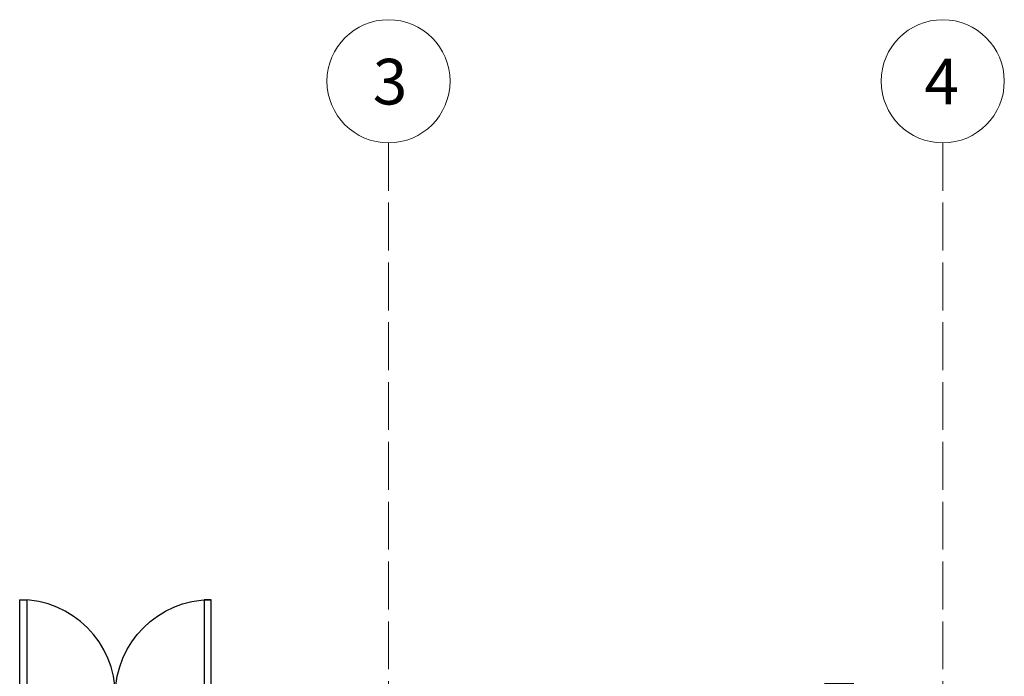
# Model space of a CAD drawing. Units: inches. Extents: x -113 to 5399, y -1393 to 3302.
# Tile 10 of 40: x 1091 to 1338, y 788 to 953. Entities that reach past the tile are written whole.
import ezdxf

# ---------------------------------------------------------------- set-up
doc = ezdxf.new("R2010")
doc.units = ezdxf.units.IN
doc.header["$MEASUREMENT"] = 0
doc.linetypes.add('ACAD_ISO02W100', pattern=[15, 12, -3])
for name, color, linetype, lineweight in [('A-ANNO-DIMS', 254, 'Continuous', 18), ('A-GRID-IDEN', 7, 'Continuous', 18), ('doors', 2, 'Continuous', 25), ('GRIDS', 7, 'ACAD_ISO02W100', 13)]:
    doc.layers.add(name, color=color, linetype=linetype, lineweight=lineweight)
doc.styles.get("Standard").update_dxf_attribs({"font": 'arial.ttf'})
doc.dimstyles.get("Standard").update_dxf_attribs({"dimtxt": 6, "dimasz": 0.18, "dimexe": 0.18, "dimexo": 0.0625, "dimgap": 0.09, "dimtad": 0, "dimtih": 1, "dimtoh": 1, "dimdec": 1, "dimzin": 0, "dimdsep": 46, "dimlunit": 4, "dimtxsty": 'Standard', "dimblk": 'ARCHTICK', "dimcen": 0.09, "dimadec": 0, "dimazin": 0, "dimtfac": 1, "dimtdec": 1, "dimtofl": 0, "dimtmove": 0, "dimatfit": 3, "dimfxl": 1, "dimtolj": 1, "dimtzin": 0, "dimarcsym": 0})

# ---------------------------------------------------------------- blocks, each defined once
blk = doc.blocks.new('*U2')
for p, q in [((0, 0), (0, -6)), ((24, 0), (24, -6))]:
    blk.add_line(p, q)
blk.add_lwpolyline([(0, 0), (0, 24), (1.75, 24), (1.75, 0)], close=True)
blk.add_arc((0, 0), 24, 0, 90)
blk = doc.blocks.new('GRID-BUBBLE-3')
blk.add_circle((0, 0), 15.44)
blk.add_text('3', height=11.45).set_placement((-3.95, -5.82))
blk = doc.blocks.new('GRID-BUBBLE-4')
blk.add_circle((0, 0), 15.44)
blk.add_text('4', height=11.45).set_placement((-4.57, -5.82))
blk = doc.blocks.new('_ArchTick')
at = {"color": 0, "linetype": 'ByBlock', "const_width": 0.15}
blk.add_lwpolyline([(-0.5, -0.5), (0.5, 0.5)], dxfattribs=at)
blk = doc.blocks.new('*D174')
at = {"layer": 'A-ANNO-DIMS', "color": 0, "lineweight": -2, "transparency": 16777216}
for p, q in [((1293.11, 786.53), (1300.43, 786.53)), ((1300.25, 786.53), (1300.25, 785.19)), ((1300.25, 777.53), (1300.25, 778.88)), ((1293.11, 777.53), (1300.43, 777.53))]:
    blk.add_line(p, q, dxfattribs=at)
at = {"layer": 'Defpoints', "color": 0, "transparency": 16777216}
for p in [(1293.05, 786.53), (1300.25, 786.53), (1293.05, 777.53)]:
    blk.add_point(p, dxfattribs=at)
at = {"layer": 'A-ANNO-DIMS', "color": 0, "lineweight": -2, "transparency": 16777216, "xscale": 0.18, "yscale": 0.18, "zscale": 0.18}
for p, rotation in [((1300.25, 786.53), 90), ((1300.25, 777.53), 270)]:
    blk.add_blockref('_ArchTick', p, dxfattribs=dict(at, rotation=rotation))
at = {"layer": 'A-ANNO-DIMS', "color": 0, "transparency": 16777216, "insert": (1300.25, 782.03), "char_height": 6, "attachment_point": 5}
blk.add_mtext('\\A1;0\'-9" TYP.', dxfattribs=at)

msp = doc.modelspace()

# ---------------------------------------------------------------- linework, layer by layer
at = {"layer": 'GRIDS'}
for p, q in [((1183.73, 922.09), (1183.73, 46.81)), ((1322.73, 922.09), (1322.73, 54.5))]:
    msp.add_line(p, q, dxfattribs=at)

# ---------------------------------------------------------------- block references
at = {"layer": 'A-GRID-IDEN'}
for name, p in [('GRID-BUBBLE-3', (1183.73, 937.53)), ('GRID-BUBBLE-4', (1322.73, 937.53))]:
    msp.add_blockref(name, p, dxfattribs=at)
at = {"layer": 'doors'}
msp.add_blockref('*U2', (1091.23, 783.53), dxfattribs=at)
at = {"layer": 'doors', "xscale": -1}
msp.add_blockref('*U2', (1139.23, 783.53), dxfattribs=at)

# ---------------------------------------------------------------- dimensions: what is measured, and where the dimension line sits
at = {"layer": 'A-ANNO-DIMS'}
dim = msp.add_linear_dim(base=(1300.25, 786.53), p1=(1293.05, 777.53), p2=(1293.05, 786.53), angle=90, text='<> TYP.', dimstyle='Standard', override={"dimdec": 1, "dimlfac": 1, "dimrnd": 0, "dimzin": 1, "dimdsep": 46, "dimlunit": 4, "dimfrac": 2}, dxfattribs=at)
dim.commit()
dim.dimension.update_dxf_attribs({"geometry": '*D174', "text_midpoint": (1300.25, 782.03)})

doc.saveas('drawing.dxf')
